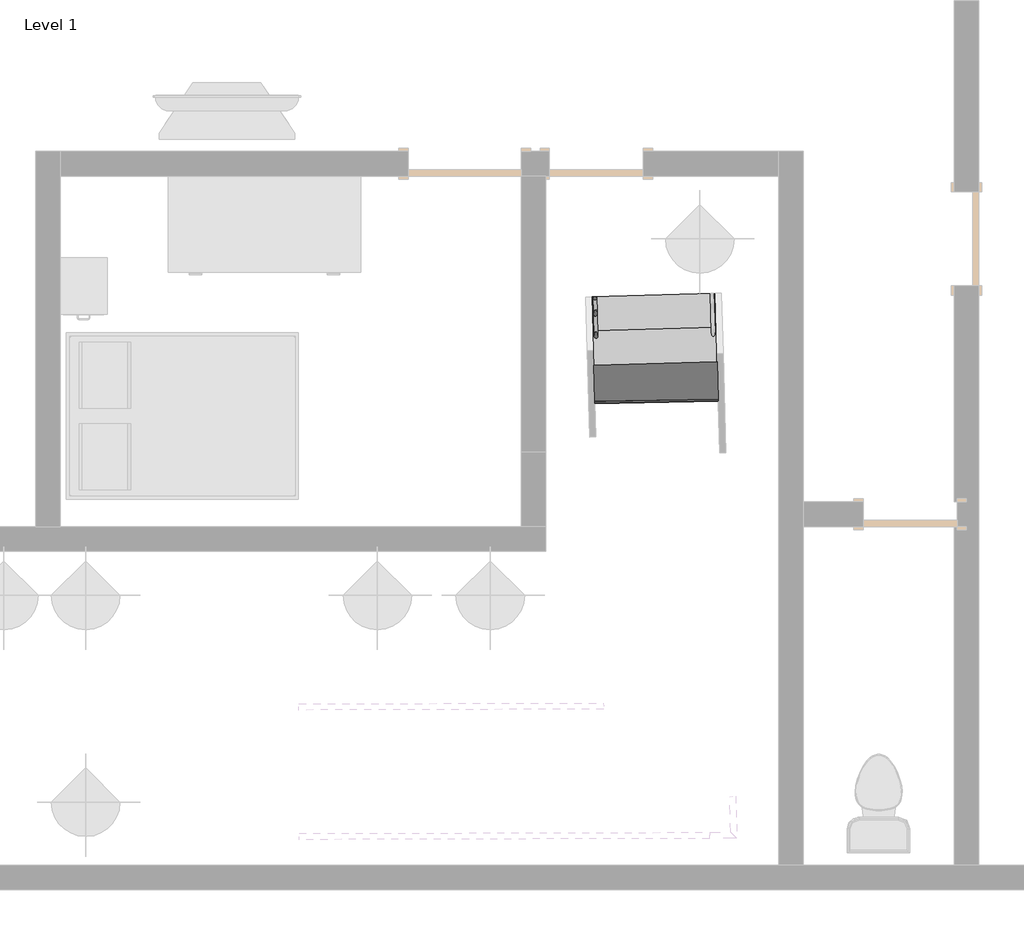
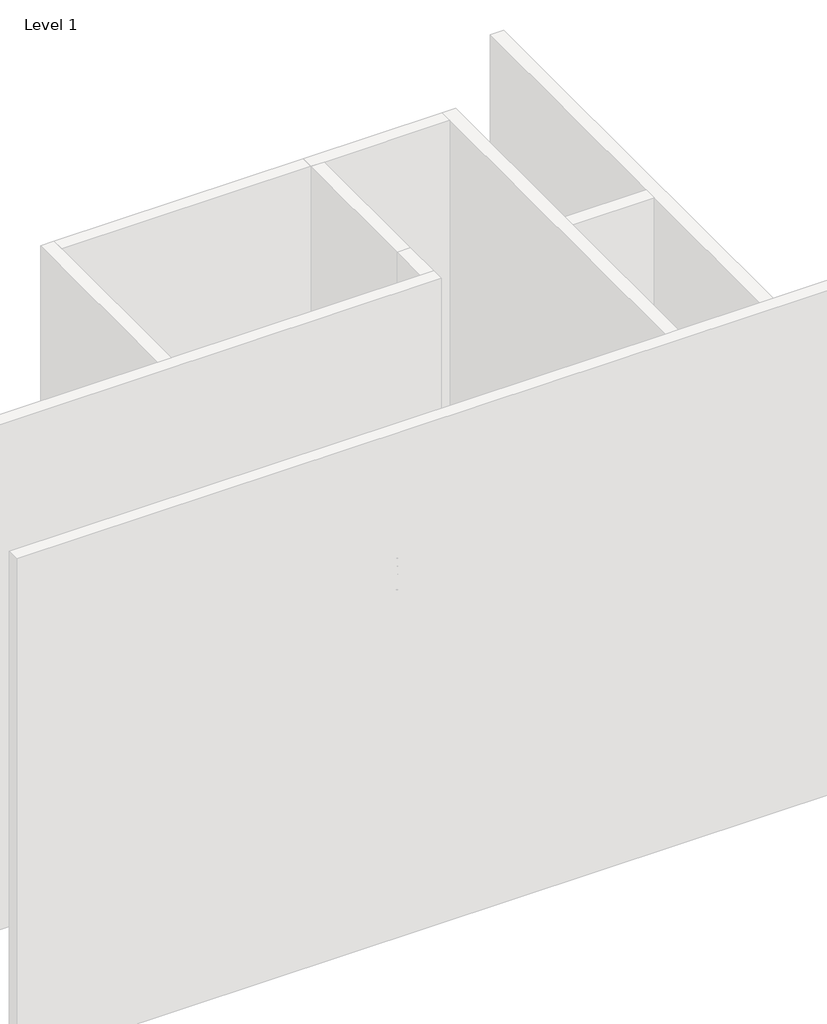
# One storey, part 3 of 4: 1 railing, 1 stair flight.
"""IFC4 building model written with IfcOpenShell, lengths in millimetres."""

from ifc_helpers import new_model, si_unit, point, frame, frame_2d, origin, place, context, project, spatial, circle_curve, ellipse_curve, trimmed, segment, composite_curve, outline, extrude, transform, mapped, element, save
from ifc_brep_helpers import plane_surface, cylinder_surface, advanced_brep
from components import stair_flight_50mm_tread_25mm_nosing_13mm_riser_f5a85d6c

model = new_model("IFC4")

# Units and contexts
model_context = context("Model", 3, world=origin())
ifc_project = project(units=[si_unit("LENGTHUNIT", "METRE", prefix="MILLI")], contexts=[model_context])

# Site, building, storey
site = spatial("IfcSite", under=ifc_project)
building = spatial("IfcBuilding", under=site)
storey = spatial("IfcBuildingStorey", under=building, Name="Level 1", Elevation=0.0)

# Railing
placement = place(None, origin())
element("IfcRailing", 1, ObjectType="900mm Pipe", at=placement, inside=storey, context=model_context, shape_type="SolidModel", body=[
    advanced_brep(
    [(2318.5093829, 1967.3130446, 1728.2894205), (2358.4929319, 1968.4601289, 1728.2894205), (2415.1133853, -1399.9817421, 4066.0870016), (2455.0969344, -1398.8346579, 4066.0870016)],
    [
        (0, 1, ellipse_curve(frame((2338.5011574, 1967.8865867, 1728.2894205), z_axis=(-0.028677106690059493, 0.9995887272032868, 0.0), x_axis=(0.0, 0.0, -1.0)), 24.3442691, 20.0)),
        (1, 0, ellipse_curve(frame((2338.5011574, 1967.8865867, 1728.2894205), z_axis=(-0.028677106690059493, 0.9995887272032868, 0.0), x_axis=(0.0, 0.0, -1.0)), 24.3442691, 20.0)),
        (2, 3, ellipse_curve(frame((2435.1051599, -1399.4082, 4066.0870016), z_axis=(0.013294885679998605, -0.46341557392153737, 0.8860413375580894), x_axis=(-0.025409101968956467, 0.885676932859188, 0.463606242557488)), 22.5723103, 20.0)),
        (3, 2, ellipse_curve(frame((2435.1051599, -1399.4082, 4066.0870016), z_axis=(0.013294885679998605, -0.46341557392153737, 0.8860413375580894), x_axis=(-0.025409101968956467, 0.885676932859188, 0.463606242557488)), 22.5723103, 20.0)),
        (0, 2),
        (3, 1),
    ],
    [
        plane_surface(frame((2338.5011574, 1967.8865867, 1752.6336896), z_axis=(-0.028677106690059493, 0.9995887272032868, 0.0), x_axis=(0.9995887272032868, 0.028677106690059493, 0.0))),
        plane_surface(frame((2434.5316177, -1379.4164255, 4076.5516656), z_axis=(0.013294885679998605, -0.46341557392153737, 0.8860413375580894), x_axis=(0.9999116191017864, 0.006161601645505646, -0.01178085949353162))),
        cylinder_surface(frame((2338.8281559, 1956.4885063, 1736.2027178), z_axis=(-0.023559636581175762, 0.8212107099253749, -0.5701385037234595), x_axis=(0.999588727203287, 0.028677106690059496, 0.0)), 20.0),
    ],
    [
        (0, [[1, 2]]),
        (1, [[3, 4]]),
        (2, [[-1, 5, -4, 6]]),
        (2, [[-2, -6, -3, -5]]),
    ],
),
    advanced_brep(
    [(2415.2157347, -1403.5493025, 4064.2195676), (2455.1992838, -1402.4022182, 4064.2195676), (2415.2157347, -1403.5493025, 4120.8684951), (2455.1992838, -1402.4022182, 4141.2378675)],
    [
        (0, 1, ellipse_curve(frame((2435.2075093, -1402.9757604, 4064.2195676), z_axis=(-0.013294885679998605, 0.46341557392153737, -0.8860413375580894), x_axis=(0.02540910196895648, -0.8856769328591886, -0.46360624255748706)), 22.5723103, 20.0)),
        (1, 0, ellipse_curve(frame((2435.2075093, -1402.9757604, 4064.2195676), z_axis=(-0.013294885679998605, 0.46341557392153737, -0.8860413375580894), x_axis=(0.02540910196895648, -0.8856769328591886, -0.46360624255748706)), 22.5723103, 20.0)),
        (2, 3, ellipse_curve(frame((2435.2075093, -1402.9757604, 4131.0531813), z_axis=(-0.4539050357854136, -0.0012028713064138657, 0.8910492531781073), x_axis=(-0.8910461243784461, -0.002361317304725111, -0.4539066296175206)), 22.4454484, 20.0)),
        (3, 2, ellipse_curve(frame((2435.2075093, -1402.9757604, 4131.0531813), z_axis=(-0.4539050357854136, -0.0012028713064138657, 0.8910492531781073), x_axis=(-0.8910461243784461, -0.002361317304725111, -0.4539066296175206)), 22.4454484, 20.0)),
        (0, 2),
        (3, 1),
    ],
    [
        plane_surface(frame((2435.1051599, -1399.4082, 4066.0870016), z_axis=(-0.013294885679998605, 0.46341557392153737, -0.8860413375580894), x_axis=(0.9999116191017864, 0.006161601645505646, -0.01178085949353162))),
        plane_surface(frame((2435.1051599, -1399.4082, 4131.00586), z_axis=(-0.4539050357854136, -0.0012028713064138657, 0.8910492531781073), x_axis=(0.8910500650853702, -0.000612748222324323, 0.45390462219608824))),
        cylinder_surface(frame((2435.2075093, -1402.9757604, 4066.0870016), z_axis=(0.0, 0.0, -1.0), x_axis=(0.9995887272032868, 0.028677106690059573, 0.0)), 20.0),
    ],
    [
        (0, [[1, 2]]),
        (1, [[3, 4]]),
        (2, [[-1, 5, -4, 6]]),
        (2, [[-2, -6, -3, -5]]),
    ],
),
    advanced_brep(
    [(2435.052159, -1379.4082702, 4131.00586), (2435.1581607, -1419.4081298, 4131.00586), (-60.3127324, -1386.0211134, 5944.7187793), (-60.2067307, -1426.020973, 5944.7187793)],
    [
        (0, 1, ellipse_curve(frame((2435.1051599, -1399.4082, 4131.00586), z_axis=(0.4539050357854136, 0.0012028713064138657, -0.8910492531781073), x_axis=(0.8910461243784458, 0.002361317304725109, 0.4539066296175212)), 22.4454484, 20.0)),
        (1, 0, ellipse_curve(frame((2435.1051599, -1399.4082, 4131.00586), z_axis=(0.4539050357854136, 0.0012028713064138657, -0.8910492531781073), x_axis=(0.8910461243784458, 0.002361317304725109, 0.4539066296175212)), 22.4454484, 20.0)),
        (2, 3, ellipse_curve(frame((-60.2597316, -1406.0210432, 5944.7187793), z_axis=(-0.9999964886344385, -0.0026500412814528056, 0.0), x_axis=(0.0, 0.0, -1.0)), 24.7247417, 20.0)),
        (3, 2, ellipse_curve(frame((-60.2597316, -1406.0210432, 5944.7187793), z_axis=(-0.9999964886344385, -0.0026500412814528056, 0.0), x_axis=(0.0, 0.0, -1.0)), 24.7247417, 20.0)),
        (0, 2),
        (3, 1),
    ],
    [
        plane_surface(frame((2455.1050896, -1399.3551992, 4141.1939978), z_axis=(0.4539050357854136, 0.0012028713064138657, -0.8910492531781073), x_axis=(0.8910500650853702, -0.000612748222324323, 0.45390462219608824))),
        plane_surface(frame((-60.2597316, -1406.0210432, 5969.443521), z_axis=(-0.9999964886344385, -0.0026500412814528056, 0.0), x_axis=(0.0026500412814528056, -0.9999964886344385, 0.0))),
        cylinder_surface(frame((2443.3463801, -1399.3863604, 4125.0158713), z_axis=(0.8089034863007496, 0.0021436351584947526, -0.5879375431785253), x_axis=(0.0026500412814528056, -0.9999964886344385, 0.0)), 20.0),
    ],
    [
        (0, [[1, 2]]),
        (1, [[3, 4]]),
        (2, [[-1, 5, -4, 6]]),
        (2, [[-2, -6, -3, -5]]),
    ],
),
    advanced_brep(
    [(2353.4949883, 1968.3167433, 1609.3754878), (2323.5073265, 1967.4564301, 1609.3754878), (2449.6798883, -1384.3695236, 3937.0308733), (2419.6698266, -1384.4490517, 3936.488801)],
    [
        (0, 1, ellipse_curve(frame((2338.5011574, 1967.8865867, 1609.3754878), z_axis=(-0.028677106690059493, 0.9995887272032868, 0.0), x_axis=(0.0, 0.0, -1.0)), 18.2582019, 15.0)),
        (1, 0, ellipse_curve(frame((2338.5011574, 1967.8865867, 1609.3754878), z_axis=(-0.028677106690059493, 0.9995887272032868, 0.0), x_axis=(0.0, 0.0, -1.0)), 18.2582019, 15.0)),
        (2, 3, ellipse_curve(frame((2434.6748575, -1384.4092877, 3936.7598372), z_axis=(0.0026500412814528056, -0.9999964886344385, 0.0), x_axis=(-0.037478985760625305, -9.93212082056486e-05, -0.9992974110652206)), 18.2643896, 15.0)),
        (3, 2, ellipse_curve(frame((2434.6748575, -1384.4092877, 3936.7598372), z_axis=(0.0026500412814528056, -0.9999964886344385, 0.0), x_axis=(-0.037478985760625305, -9.93212082056486e-05, -0.9992974110652206)), 18.2643896, 15.0)),
        (0, 2),
        (3, 1),
    ],
    [
        plane_surface(frame((2338.5011574, 1967.8865867, 1627.6336896), z_axis=(-0.028677106690059493, 0.9995887272032868, 0.0), x_axis=(0.9995887272032868, 0.028677106690059493, 0.0))),
        plane_surface(frame((2434.6748575, -1384.4092877, 3955.018039), z_axis=(0.0026500412814528056, -0.9999964886344385, 0.0), x_axis=(0.9999964886344385, 0.0026500412814528056, 0.0))),
        cylinder_surface(frame((2338.7464062, 1959.3380264, 1615.3104608), z_axis=(-0.023559636581175762, 0.8212107099253748, -0.5701385037234593), x_axis=(-0.9995887272032868, -0.028677106690059496, 0.0)), 15.0),
    ],
    [
        (0, [[1, 2]]),
        (1, [[3, 4]]),
        (2, [[-1, 5, -4, 6]]),
        (2, [[-2, -6, -3, -5]]),
    ],
),
    advanced_brep(
    [(2450.5404931, -1414.3673483, 4000.9970318), (2449.6798883, -1384.3695236, 4001.5647634), (-60.219981, -1421.0209905, 5825.8999647), (-60.2994822, -1391.0210959, 5825.8999647)],
    [
        (0, 1, ellipse_curve(frame((2450.1101907, -1399.3684359, 4001.2808976), z_axis=(0.9995887272032868, 0.028677106690059493, 0.0), x_axis=(0.0010262798280310235, -0.03577270741234457, -0.9993594249088289)), 18.5498407, 15.0)),
        (1, 0, ellipse_curve(frame((2450.1101907, -1399.3684359, 4001.2808976), z_axis=(0.9995887272032868, 0.028677106690059493, 0.0), x_axis=(0.0010262798280310235, -0.03577270741234457, -0.9993594249088289)), 18.5498407, 15.0)),
        (2, 3, ellipse_curve(frame((-60.2597316, -1406.0210432, 5825.8999647), z_axis=(-0.9999964886344385, -0.0026500412814528056, 0.0), x_axis=(0.0, 0.0, -1.0)), 18.5435563, 15.0)),
        (3, 2, ellipse_curve(frame((-60.2597316, -1406.0210432, 5825.8999647), z_axis=(-0.9999964886344385, -0.0026500412814528056, 0.0), x_axis=(0.0, 0.0, -1.0)), 18.5435563, 15.0)),
        (0, 2),
        (3, 1),
    ],
    [
        plane_surface(frame((2450.1101907, -1399.3684359, 4019.8244539), z_axis=(0.9995887272032868, 0.028677106690059493, 0.0), x_axis=(0.028677106690059493, -0.9995887272032868, 0.0))),
        plane_surface(frame((-60.2597316, -1406.0210432, 5844.443521), z_axis=(-0.9999964886344385, -0.0026500412814528056, 0.0), x_axis=(0.0026500412814528056, -0.9999964886344385, 0.0))),
        cylinder_surface(frame((2441.2911585, -1399.3918068, 4007.690859), z_axis=(0.8089034863007496, 0.0021436351584947526, -0.5879375431785254), x_axis=(-0.0026500412814528056, 0.9999964886344385, 0.0)), 15.0),
    ],
    [
        (0, [[1, 2]]),
        (1, [[3, 4]]),
        (2, [[-1, 5, -4, 6]]),
        (2, [[-2, -6, -3, -5]]),
    ],
),
    advanced_brep(
    [(2353.4949883, 1968.3167433, 1484.3754878), (2323.5073265, 1967.4564301, 1484.3754878), (2449.6798883, -1384.3695236, 3812.0308733), (2419.6698266, -1384.4490517, 3811.488801)],
    [
        (0, 1, ellipse_curve(frame((2338.5011574, 1967.8865867, 1484.3754878), z_axis=(-0.028677106690059493, 0.9995887272032868, 0.0), x_axis=(0.0, 0.0, -1.0)), 18.2582019, 15.0)),
        (1, 0, ellipse_curve(frame((2338.5011574, 1967.8865867, 1484.3754878), z_axis=(-0.028677106690059493, 0.9995887272032868, 0.0), x_axis=(0.0, 0.0, -1.0)), 18.2582019, 15.0)),
        (2, 3, ellipse_curve(frame((2434.6748575, -1384.4092877, 3811.7598372), z_axis=(0.0026500412814528056, -0.9999964886344385, 0.0), x_axis=(-0.037478985760625305, -9.93212082056486e-05, -0.9992974110652206)), 18.2643896, 15.0)),
        (3, 2, ellipse_curve(frame((2434.6748575, -1384.4092877, 3811.7598372), z_axis=(0.0026500412814528056, -0.9999964886344385, 0.0), x_axis=(-0.037478985760625305, -9.93212082056486e-05, -0.9992974110652206)), 18.2643896, 15.0)),
        (0, 2),
        (3, 1),
    ],
    [
        plane_surface(frame((2338.5011574, 1967.8865867, 1502.6336896), z_axis=(-0.028677106690059493, 0.9995887272032868, 0.0), x_axis=(0.9995887272032868, 0.028677106690059493, 0.0))),
        plane_surface(frame((2434.6748575, -1384.4092877, 3830.018039), z_axis=(0.0026500412814528056, -0.9999964886344385, 0.0), x_axis=(0.9999964886344385, 0.0026500412814528056, 0.0))),
        cylinder_surface(frame((2338.7464062, 1959.3380264, 1490.3104608), z_axis=(-0.023559636581175762, 0.8212107099253748, -0.5701385037234593), x_axis=(-0.9995887272032868, -0.028677106690059496, 0.0)), 15.0),
    ],
    [
        (0, [[1, 2]]),
        (1, [[3, 4]]),
        (2, [[-1, 5, -4, 6]]),
        (2, [[-2, -6, -3, -5]]),
    ],
),
    advanced_brep(
    [(2450.5404931, -1414.3673483, 3875.9970318), (2449.6798883, -1384.3695236, 3876.5647634), (-60.219981, -1421.0209905, 5700.8999647), (-60.2994822, -1391.0210959, 5700.8999647)],
    [
        (0, 1, ellipse_curve(frame((2450.1101907, -1399.3684359, 3876.2808976), z_axis=(0.9995887272032868, 0.028677106690059493, 0.0), x_axis=(0.001026279828031024, -0.03577270741234459, -0.9993594249088289)), 18.5498407, 15.0)),
        (1, 0, ellipse_curve(frame((2450.1101907, -1399.3684359, 3876.2808976), z_axis=(0.9995887272032868, 0.028677106690059493, 0.0), x_axis=(0.001026279828031024, -0.03577270741234459, -0.9993594249088289)), 18.5498407, 15.0)),
        (2, 3, ellipse_curve(frame((-60.2597316, -1406.0210432, 5700.8999647), z_axis=(-0.9999964886344385, -0.0026500412814528056, 0.0), x_axis=(0.0, 0.0, -0.9999999999999999)), 18.5435563, 15.0)),
        (3, 2, ellipse_curve(frame((-60.2597316, -1406.0210432, 5700.8999647), z_axis=(-0.9999964886344385, -0.0026500412814528056, 0.0), x_axis=(0.0, 0.0, -0.9999999999999999)), 18.5435563, 15.0)),
        (0, 2),
        (3, 1),
    ],
    [
        plane_surface(frame((2450.1101907, -1399.3684359, 3894.8244539), z_axis=(0.9995887272032868, 0.028677106690059493, 0.0), x_axis=(0.028677106690059493, -0.9995887272032868, 0.0))),
        plane_surface(frame((-60.2597316, -1406.0210432, 5719.443521), z_axis=(-0.9999964886344385, -0.0026500412814528056, 0.0), x_axis=(0.0026500412814528056, -0.9999964886344385, 0.0))),
        cylinder_surface(frame((2441.2911585, -1399.3918068, 3882.690859), z_axis=(0.8089034863007497, 0.0021436351584947534, -0.5879375431785252), x_axis=(-0.002650041281452806, 0.9999964886344385, 0.0)), 15.0),
    ],
    [
        (0, [[1, 2]]),
        (1, [[3, 4]]),
        (2, [[-1, 5, -4, 6]]),
        (2, [[-2, -6, -3, -5]]),
    ],
),
    advanced_brep(
    [(2353.4949883, 1968.3167433, 1359.3754878), (2323.5073265, 1967.4564301, 1359.3754878), (2449.6798883, -1384.3695236, 3687.0308733), (2419.6698266, -1384.4490517, 3686.488801)],
    [
        (0, 1, ellipse_curve(frame((2338.5011574, 1967.8865867, 1359.3754878), z_axis=(-0.028677106690059493, 0.9995887272032868, 0.0), x_axis=(0.0, 0.0, -1.0)), 18.2582019, 15.0)),
        (1, 0, ellipse_curve(frame((2338.5011574, 1967.8865867, 1359.3754878), z_axis=(-0.028677106690059493, 0.9995887272032868, 0.0), x_axis=(0.0, 0.0, -1.0)), 18.2582019, 15.0)),
        (2, 3, ellipse_curve(frame((2434.6748575, -1384.4092877, 3686.7598372), z_axis=(0.0026500412814528056, -0.9999964886344385, 0.0), x_axis=(-0.03747898576062528, -9.932120820564857e-05, -0.9992974110652205)), 18.2643896, 15.0)),
        (3, 2, ellipse_curve(frame((2434.6748575, -1384.4092877, 3686.7598372), z_axis=(0.0026500412814528056, -0.9999964886344385, 0.0), x_axis=(-0.03747898576062528, -9.932120820564857e-05, -0.9992974110652205)), 18.2643896, 15.0)),
        (0, 2),
        (3, 1),
    ],
    [
        plane_surface(frame((2338.5011574, 1967.8865867, 1377.6336896), z_axis=(-0.028677106690059493, 0.9995887272032868, 0.0), x_axis=(0.9995887272032868, 0.028677106690059493, 0.0))),
        plane_surface(frame((2434.6748575, -1384.4092877, 3705.018039), z_axis=(0.0026500412814528056, -0.9999964886344385, 0.0), x_axis=(0.9999964886344385, 0.0026500412814528056, 0.0))),
        cylinder_surface(frame((2338.7464062, 1959.3380264, 1365.3104608), z_axis=(-0.023559636581175762, 0.8212107099253749, -0.5701385037234595), x_axis=(-0.999588727203287, -0.028677106690059496, 0.0)), 15.0),
    ],
    [
        (0, [[1, 2]]),
        (1, [[3, 4]]),
        (2, [[-1, 5, -4, 6]]),
        (2, [[-2, -6, -3, -5]]),
    ],
),
    advanced_brep(
    [(2450.5404931, -1414.3673483, 3750.9970318), (2449.6798883, -1384.3695236, 3751.5647634), (-60.219981, -1421.0209905, 5575.8999647), (-60.2994822, -1391.0210959, 5575.8999647)],
    [
        (0, 1, ellipse_curve(frame((2450.1101907, -1399.3684359, 3751.2808976), z_axis=(0.9995887272032868, 0.028677106690059493, 0.0), x_axis=(0.001026279828031024, -0.03577270741234459, -0.9993594249088289)), 18.5498407, 15.0)),
        (1, 0, ellipse_curve(frame((2450.1101907, -1399.3684359, 3751.2808976), z_axis=(0.9995887272032868, 0.028677106690059493, 0.0), x_axis=(0.001026279828031024, -0.03577270741234459, -0.9993594249088289)), 18.5498407, 15.0)),
        (2, 3, ellipse_curve(frame((-60.2597316, -1406.0210432, 5575.8999647), z_axis=(-0.9999964886344385, -0.0026500412814528056, 0.0), x_axis=(0.0, 0.0, -0.9999999999999999)), 18.5435563, 15.0)),
        (3, 2, ellipse_curve(frame((-60.2597316, -1406.0210432, 5575.8999647), z_axis=(-0.9999964886344385, -0.0026500412814528056, 0.0), x_axis=(0.0, 0.0, -0.9999999999999999)), 18.5435563, 15.0)),
        (0, 2),
        (3, 1),
    ],
    [
        plane_surface(frame((2450.1101907, -1399.3684359, 3769.8244539), z_axis=(0.9995887272032868, 0.028677106690059493, 0.0), x_axis=(0.028677106690059493, -0.9995887272032868, 0.0))),
        plane_surface(frame((-60.2597316, -1406.0210432, 5594.443521), z_axis=(-0.9999964886344385, -0.0026500412814528056, 0.0), x_axis=(0.0026500412814528056, -0.9999964886344385, 0.0))),
        cylinder_surface(frame((2441.2911585, -1399.3918068, 3757.690859), z_axis=(0.8089034863007497, 0.0021436351584947534, -0.5879375431785252), x_axis=(-0.002650041281452806, 0.9999964886344385, 0.0)), 15.0),
    ],
    [
        (0, [[1, 2]]),
        (1, [[3, 4]]),
        (2, [[-1, 5, -4, 6]]),
        (2, [[-2, -6, -3, -5]]),
    ],
),
    advanced_brep(
    [(2353.4949883, 1968.3167433, 1234.3754878), (2323.5073265, 1967.4564301, 1234.3754878), (2449.6798883, -1384.3695236, 3562.0308733), (2419.6698266, -1384.4490517, 3561.488801)],
    [
        (0, 1, ellipse_curve(frame((2338.5011574, 1967.8865867, 1234.3754878), z_axis=(-0.028677106690059493, 0.9995887272032868, 0.0), x_axis=(0.0, 0.0, -1.0)), 18.2582019, 15.0)),
        (1, 0, ellipse_curve(frame((2338.5011574, 1967.8865867, 1234.3754878), z_axis=(-0.028677106690059493, 0.9995887272032868, 0.0), x_axis=(0.0, 0.0, -1.0)), 18.2582019, 15.0)),
        (2, 3, ellipse_curve(frame((2434.6748575, -1384.4092877, 3561.7598372), z_axis=(0.0026500412814528056, -0.9999964886344385, 0.0), x_axis=(-0.037478985760625305, -9.93212082056486e-05, -0.9992974110652206)), 18.2643896, 15.0)),
        (3, 2, ellipse_curve(frame((2434.6748575, -1384.4092877, 3561.7598372), z_axis=(0.0026500412814528056, -0.9999964886344385, 0.0), x_axis=(-0.037478985760625305, -9.93212082056486e-05, -0.9992974110652206)), 18.2643896, 15.0)),
        (0, 2),
        (3, 1),
    ],
    [
        plane_surface(frame((2338.5011574, 1967.8865867, 1252.6336896), z_axis=(-0.028677106690059493, 0.9995887272032868, 0.0), x_axis=(0.9995887272032868, 0.028677106690059493, 0.0))),
        plane_surface(frame((2434.6748575, -1384.4092877, 3580.018039), z_axis=(0.0026500412814528056, -0.9999964886344385, 0.0), x_axis=(0.9999964886344385, 0.0026500412814528056, 0.0))),
        cylinder_surface(frame((2338.7464062, 1959.3380264, 1240.3104608), z_axis=(-0.023559636581175762, 0.8212107099253748, -0.5701385037234593), x_axis=(-0.9995887272032868, -0.028677106690059496, 0.0)), 15.0),
    ],
    [
        (0, [[1, 2]]),
        (1, [[3, 4]]),
        (2, [[-1, 5, -4, 6]]),
        (2, [[-2, -6, -3, -5]]),
    ],
),
    advanced_brep(
    [(2450.5404931, -1414.3673483, 3625.9970318), (2449.6798883, -1384.3695236, 3626.5647634), (-60.219981, -1421.0209905, 5450.8999647), (-60.2994822, -1391.0210959, 5450.8999647)],
    [
        (0, 1, ellipse_curve(frame((2450.1101907, -1399.3684359, 3626.2808976), z_axis=(0.9995887272032868, 0.028677106690059493, 0.0), x_axis=(0.0010262798280310237, -0.03577270741234458, -0.999359424908829)), 18.5498407, 15.0)),
        (1, 0, ellipse_curve(frame((2450.1101907, -1399.3684359, 3626.2808976), z_axis=(0.9995887272032868, 0.028677106690059493, 0.0), x_axis=(0.0010262798280310237, -0.03577270741234458, -0.999359424908829)), 18.5498407, 15.0)),
        (2, 3, ellipse_curve(frame((-60.2597316, -1406.0210432, 5450.8999647), z_axis=(-0.9999964886344385, -0.0026500412814528056, 0.0), x_axis=(0.0, 0.0, -1.0)), 18.5435563, 15.0)),
        (3, 2, ellipse_curve(frame((-60.2597316, -1406.0210432, 5450.8999647), z_axis=(-0.9999964886344385, -0.0026500412814528056, 0.0), x_axis=(0.0, 0.0, -1.0)), 18.5435563, 15.0)),
        (0, 2),
        (3, 1),
    ],
    [
        plane_surface(frame((2450.1101907, -1399.3684359, 3644.8244539), z_axis=(0.9995887272032868, 0.028677106690059493, 0.0), x_axis=(0.028677106690059493, -0.9995887272032868, 0.0))),
        plane_surface(frame((-60.2597316, -1406.0210432, 5469.443521), z_axis=(-0.9999964886344385, -0.0026500412814528056, 0.0), x_axis=(0.0026500412814528056, -0.9999964886344385, 0.0))),
        cylinder_surface(frame((2441.2911585, -1399.3918068, 3632.690859), z_axis=(0.8089034863007496, 0.0021436351584947526, -0.5879375431785253), x_axis=(-0.0026500412814528056, 0.9999964886344385, 0.0)), 15.0),
    ],
    [
        (0, [[1, 2]]),
        (1, [[3, 4]]),
        (2, [[-1, 5, -4, 6]]),
        (2, [[-2, -6, -3, -5]]),
    ],
),
    advanced_brep(
    [(2353.4949883, 1968.3167433, 1109.3754878), (2323.5073265, 1967.4564301, 1109.3754878), (2449.6798883, -1384.3695236, 3437.0308733), (2419.6698266, -1384.4490517, 3436.488801)],
    [
        (0, 1, ellipse_curve(frame((2338.5011574, 1967.8865867, 1109.3754878), z_axis=(-0.028677106690059493, 0.9995887272032868, 0.0), x_axis=(0.0, 0.0, -1.0)), 18.2582019, 15.0)),
        (1, 0, ellipse_curve(frame((2338.5011574, 1967.8865867, 1109.3754878), z_axis=(-0.028677106690059493, 0.9995887272032868, 0.0), x_axis=(0.0, 0.0, -1.0)), 18.2582019, 15.0)),
        (2, 3, ellipse_curve(frame((2434.6748575, -1384.4092877, 3436.7598372), z_axis=(0.0026500412814528056, -0.9999964886344385, 0.0), x_axis=(-0.037478985760625305, -9.93212082056486e-05, -0.9992974110652206)), 18.2643896, 15.0)),
        (3, 2, ellipse_curve(frame((2434.6748575, -1384.4092877, 3436.7598372), z_axis=(0.0026500412814528056, -0.9999964886344385, 0.0), x_axis=(-0.037478985760625305, -9.93212082056486e-05, -0.9992974110652206)), 18.2643896, 15.0)),
        (0, 2),
        (3, 1),
    ],
    [
        plane_surface(frame((2338.5011574, 1967.8865867, 1127.6336896), z_axis=(-0.028677106690059493, 0.9995887272032868, 0.0), x_axis=(0.9995887272032868, 0.028677106690059493, 0.0))),
        plane_surface(frame((2434.6748575, -1384.4092877, 3455.018039), z_axis=(0.0026500412814528056, -0.9999964886344385, 0.0), x_axis=(0.9999964886344385, 0.0026500412814528056, 0.0))),
        cylinder_surface(frame((2338.7464062, 1959.3380264, 1115.3104608), z_axis=(-0.023559636581175762, 0.8212107099253748, -0.5701385037234593), x_axis=(-0.9995887272032868, -0.028677106690059496, 0.0)), 15.0),
    ],
    [
        (0, [[1, 2]]),
        (1, [[3, 4]]),
        (2, [[-1, 5, -4, 6]]),
        (2, [[-2, -6, -3, -5]]),
    ],
),
    advanced_brep(
    [(2450.5404931, -1414.3673483, 3500.9970318), (2449.6798883, -1384.3695236, 3501.5647634), (-60.219981, -1421.0209905, 5325.8999647), (-60.2994822, -1391.0210959, 5325.8999647)],
    [
        (0, 1, ellipse_curve(frame((2450.1101907, -1399.3684359, 3501.2808976), z_axis=(0.9995887272032868, 0.028677106690059493, 0.0), x_axis=(0.0010262798280310235, -0.03577270741234457, -0.9993594249088289)), 18.5498407, 15.0)),
        (1, 0, ellipse_curve(frame((2450.1101907, -1399.3684359, 3501.2808976), z_axis=(0.9995887272032868, 0.028677106690059493, 0.0), x_axis=(0.0010262798280310235, -0.03577270741234457, -0.9993594249088289)), 18.5498407, 15.0)),
        (2, 3, ellipse_curve(frame((-60.2597316, -1406.0210432, 5325.8999647), z_axis=(-0.9999964886344385, -0.0026500412814528056, 0.0), x_axis=(0.0, 0.0, -1.0)), 18.5435563, 15.0)),
        (3, 2, ellipse_curve(frame((-60.2597316, -1406.0210432, 5325.8999647), z_axis=(-0.9999964886344385, -0.0026500412814528056, 0.0), x_axis=(0.0, 0.0, -1.0)), 18.5435563, 15.0)),
        (0, 2),
        (3, 1),
    ],
    [
        plane_surface(frame((2450.1101907, -1399.3684359, 3519.8244539), z_axis=(0.9995887272032868, 0.028677106690059493, 0.0), x_axis=(0.028677106690059493, -0.9995887272032868, 0.0))),
        plane_surface(frame((-60.2597316, -1406.0210432, 5344.443521), z_axis=(-0.9999964886344385, -0.0026500412814528056, 0.0), x_axis=(0.0026500412814528056, -0.9999964886344385, 0.0))),
        cylinder_surface(frame((2441.2911585, -1399.3918068, 3507.690859), z_axis=(0.8089034863007496, 0.0021436351584947526, -0.5879375431785254), x_axis=(-0.0026500412814528056, 0.9999964886344385, 0.0)), 15.0),
    ],
    [
        (0, [[1, 2]]),
        (1, [[3, 4]]),
        (2, [[-1, 5, -4, 6]]),
        (2, [[-2, -6, -3, -5]]),
    ],
),
    advanced_brep(
    [(2353.4949883, 1968.3167433, 984.3754878), (2323.5073265, 1967.4564301, 984.3754878), (2449.6798883, -1384.3695236, 3312.0308733), (2419.6698266, -1384.4490517, 3311.488801)],
    [
        (0, 1, ellipse_curve(frame((2338.5011574, 1967.8865867, 984.3754878), z_axis=(-0.028677106690059493, 0.9995887272032868, 0.0), x_axis=(0.0, 0.0, -1.0)), 18.2582019, 15.0)),
        (1, 0, ellipse_curve(frame((2338.5011574, 1967.8865867, 984.3754878), z_axis=(-0.028677106690059493, 0.9995887272032868, 0.0), x_axis=(0.0, 0.0, -1.0)), 18.2582019, 15.0)),
        (2, 3, ellipse_curve(frame((2434.6748575, -1384.4092877, 3311.7598372), z_axis=(0.0026500412814528056, -0.9999964886344385, 0.0), x_axis=(-0.037478985760625305, -9.93212082056486e-05, -0.9992974110652206)), 18.2643896, 15.0)),
        (3, 2, ellipse_curve(frame((2434.6748575, -1384.4092877, 3311.7598372), z_axis=(0.0026500412814528056, -0.9999964886344385, 0.0), x_axis=(-0.037478985760625305, -9.93212082056486e-05, -0.9992974110652206)), 18.2643896, 15.0)),
        (0, 2),
        (3, 1),
    ],
    [
        plane_surface(frame((2338.5011574, 1967.8865867, 1002.6336896), z_axis=(-0.028677106690059493, 0.9995887272032868, 0.0), x_axis=(0.9995887272032868, 0.028677106690059493, 0.0))),
        plane_surface(frame((2434.6748575, -1384.4092877, 3330.018039), z_axis=(0.0026500412814528056, -0.9999964886344385, 0.0), x_axis=(0.9999964886344385, 0.0026500412814528056, 0.0))),
        cylinder_surface(frame((2338.7464062, 1959.3380264, 990.3104608), z_axis=(-0.023559636581175762, 0.8212107099253748, -0.5701385037234593), x_axis=(-0.9995887272032868, -0.028677106690059496, 0.0)), 15.0),
    ],
    [
        (0, [[1, 2]]),
        (1, [[3, 4]]),
        (2, [[-1, 5, -4, 6]]),
        (2, [[-2, -6, -3, -5]]),
    ],
),
    advanced_brep(
    [(2450.5404931, -1414.3673483, 3375.9970318), (2449.6798883, -1384.3695236, 3376.5647634), (-60.219981, -1421.0209905, 5200.8999647), (-60.2994822, -1391.0210959, 5200.8999647)],
    [
        (0, 1, ellipse_curve(frame((2450.1101907, -1399.3684359, 3376.2808976), z_axis=(0.9995887272032868, 0.028677106690059493, 0.0), x_axis=(0.0010262798280310235, -0.03577270741234457, -0.9993594249088289)), 18.5498407, 15.0)),
        (1, 0, ellipse_curve(frame((2450.1101907, -1399.3684359, 3376.2808976), z_axis=(0.9995887272032868, 0.028677106690059493, 0.0), x_axis=(0.0010262798280310235, -0.03577270741234457, -0.9993594249088289)), 18.5498407, 15.0)),
        (2, 3, ellipse_curve(frame((-60.2597316, -1406.0210432, 5200.8999647), z_axis=(-0.9999964886344385, -0.0026500412814528056, 0.0), x_axis=(0.0, 0.0, -1.0)), 18.5435563, 15.0)),
        (3, 2, ellipse_curve(frame((-60.2597316, -1406.0210432, 5200.8999647), z_axis=(-0.9999964886344385, -0.0026500412814528056, 0.0), x_axis=(0.0, 0.0, -1.0)), 18.5435563, 15.0)),
        (0, 2),
        (3, 1),
    ],
    [
        plane_surface(frame((2450.1101907, -1399.3684359, 3394.8244539), z_axis=(0.9995887272032868, 0.028677106690059493, 0.0), x_axis=(0.028677106690059493, -0.9995887272032868, 0.0))),
        plane_surface(frame((-60.2597316, -1406.0210432, 5219.443521), z_axis=(-0.9999964886344385, -0.0026500412814528056, 0.0), x_axis=(0.0026500412814528056, -0.9999964886344385, 0.0))),
        cylinder_surface(frame((2441.2911585, -1399.3918068, 3382.690859), z_axis=(0.8089034863007496, 0.0021436351584947526, -0.5879375431785254), x_axis=(-0.0026500412814528056, 0.9999964886344385, 0.0)), 15.0),
    ],
    [
        (0, [[1, 2]]),
        (1, [[3, 4]]),
        (2, [[-1, 5, -4, 6]]),
        (2, [[-2, -6, -3, -5]]),
    ],
),
    advanced_brep(
    [(435.0790571, -1392.2083265, 5559.9415083), (435.0790571, -1392.2083265, 4695.6521739), (435.1453081, -1417.2082387, 4695.6521739), (435.1453081, -1417.2082387, 5559.9415083)],
    [
        (0, 1),
        (1, 2, circle_curve(frame((435.1121826, -1404.7082826, 4695.6521739), z_axis=(0.0, 0.0, 1.0), x_axis=(0.002650041281452805, -0.9999964886344386, 0.0)), 12.5)),
        (2, 3),
        (3, 0, ellipse_curve(frame((435.1121826, -1404.7082826, 5559.9415083), z_axis=(-0.5879354787148848, -0.0015580587603390356, -0.808906326666567), x_axis=(-0.8089034863007493, -0.0021436351584947512, 0.587937543178526)), 15.4529636, 12.5)),
        (0, 3, ellipse_curve(frame((435.1121826, -1404.7082826, 5559.9415083), z_axis=(-0.5879354787148848, -0.0015580587603390356, -0.808906326666567), x_axis=(-0.8089034863007493, -0.0021436351584947512, 0.587937543178526)), 15.4529636, 12.5)),
        (2, 1, circle_curve(frame((435.1121826, -1404.7082826, 4695.6521739), z_axis=(0.0, 0.0, 1.0), x_axis=(0.002650041281452805, -0.9999964886344386, 0.0)), 12.5)),
    ],
    [
        cylinder_surface(frame((435.1121826, -1404.7082826, 4595.6521739), z_axis=(0.0, 0.0, 1.0), x_axis=(0.002650041281452805, -0.9999964886344386, 0.0)), 12.5),
        plane_surface(frame((410.1785214, -1429.7744458, 5578.1122632), z_axis=(0.5879354787148848, 0.0015580587603390356, 0.808906326666567), x_axis=(-0.002650041281452805, 0.9999964886344386, 0.0))),
        plane_surface(frame((460.1783458, -1429.6419438, 4695.6521739), z_axis=(0.0, 0.0, -1.0), x_axis=(-0.002650041281452805, 0.9999964886344386, 0.0))),
    ],
    [
        (0, [[1, 2, 3, 4]]),
        (0, [[-1, 5, -3, 6]]),
        (1, [[-4, -5]]),
        (2, [[-2, -6]]),
    ],
),
    advanced_brep(
    [(1435.0755457, -1389.5582852, 4833.1113133), (1435.0755457, -1389.5582852, 4000.0), (1435.1417967, -1414.5581974, 4000.0), (1435.1417967, -1414.5581974, 4833.1113133)],
    [
        (0, 1),
        (1, 2, circle_curve(frame((1435.1086712, -1402.0582413, 4000.0), z_axis=(0.0, 0.0, 1.0), x_axis=(0.002650041281452805, -0.9999964886344386, 0.0)), 12.5)),
        (2, 3),
        (3, 0, ellipse_curve(frame((1435.1086712, -1402.0582413, 4833.1113133), z_axis=(-0.5879354787148834, -0.0015580587603390317, -0.808906326666568), x_axis=(-0.8089034863007504, -0.002143635158494754, 0.5879375431785245)), 15.4529636, 12.5)),
        (0, 3, ellipse_curve(frame((1435.1086712, -1402.0582413, 4833.1113133), z_axis=(-0.5879354787148834, -0.0015580587603390317, -0.808906326666568), x_axis=(-0.8089034863007504, -0.002143635158494754, 0.5879375431785245)), 15.4529636, 12.5)),
        (2, 1, circle_curve(frame((1435.1086712, -1402.0582413, 4000.0), z_axis=(0.0, 0.0, 1.0), x_axis=(0.002650041281452805, -0.9999964886344386, 0.0)), 12.5)),
    ],
    [
        cylinder_surface(frame((1435.1086712, -1402.0582413, 3900.0), z_axis=(0.0, 0.0, 1.0), x_axis=(0.002650041281452805, -0.9999964886344386, 0.0)), 12.5),
        plane_surface(frame((1410.17501, -1427.1244045, 4851.2820682), z_axis=(0.5879354787148834, 0.0015580587603390317, 0.808906326666568), x_axis=(-0.002650041281452805, 0.9999964886344386, 0.0))),
        plane_surface(frame((1460.1748345, -1426.9919025, 4000.0), z_axis=(0.0, 0.0, -1.0), x_axis=(-0.002650041281452805, 0.9999964886344386, 0.0))),
    ],
    [
        (0, [[1, 2, 3, 4]]),
        (0, [[-1, 5, -3, 6]]),
        (1, [[-4, -5]]),
        (2, [[-2, -6]]),
    ],
),
    advanced_brep(
    [(2412.0376184, -1031.2380587, 3785.8859287), (2412.0376184, -1031.2380587, 2782.6086957), (2437.0273366, -1030.5211311, 2782.6086957), (2437.0273366, -1030.5211311, 3785.8859287)],
    [
        (0, 1),
        (1, 2, circle_curve(frame((2424.5324775, -1030.8795949, 2782.6086957), z_axis=(0.0, 0.0, 1.0000000000000002), x_axis=(0.999588727203287, 0.028677106690059514, 0.0)), 12.5)),
        (2, 3),
        (3, 0, ellipse_curve(frame((2424.5324775, -1030.8795949, 3785.8859287), z_axis=(0.016349922699388522, -0.5699040212665187, -0.8215485905118309), x_axis=(0.02355963658117579, -0.8212107099253754, 0.5701385037234586)), 15.2151682, 12.5)),
        (0, 3, ellipse_curve(frame((2424.5324775, -1030.8795949, 3785.8859287), z_axis=(0.016349922699388522, -0.5699040212665187, -0.8215485905118309), x_axis=(0.02355963658117579, -0.8212107099253754, 0.5701385037234586)), 15.2151682, 12.5)),
        (2, 1, circle_curve(frame((2424.5324775, -1030.8795949, 2782.6086957), z_axis=(0.0, 0.0, 1.0000000000000002), x_axis=(0.999588727203287, 0.028677106690059514, 0.0)), 12.5)),
    ],
    [
        cylinder_surface(frame((2424.5324775, -1030.8795949, 2682.6086957), z_axis=(0.0, 0.0, 1.0000000000000002), x_axis=(0.999588727203287, 0.028677106690059514, 0.0)), 12.5),
        plane_surface(frame((2450.2391233, -1055.1523854, 3803.2354352), z_axis=(-0.016349922699388522, 0.5699040212665187, 0.8215485905118309), x_axis=(-0.999588727203287, -0.028677106690059514, 0.0))),
        plane_surface(frame((2448.805268, -1005.172949, 2782.6086957), z_axis=(0.0, 0.0, -1.0000000000000002), x_axis=(-0.999588727203287, -0.028677106690059514, 0.0))),
    ],
    [
        (0, [[1, 2, 3, 4]]),
        (0, [[-1, 5, -3, 6]]),
        (1, [[-4, -5]]),
        (2, [[-2, -6]]),
    ],
),
    advanced_brep(
    [(2383.3605117, -31.6493315, 3091.9056696), (2383.3605117, -31.6493315, 2086.9565217), (2408.3502299, -30.9324039, 2086.9565217), (2408.3502299, -30.9324039, 3091.9056696)],
    [
        (0, 1),
        (1, 2, circle_curve(frame((2395.8553708, -31.2908677, 2086.9565217), z_axis=(0.0, 0.0, 1.0000000000000002), x_axis=(0.999588727203287, 0.028677106690059514, 0.0)), 12.5)),
        (2, 3),
        (3, 0, ellipse_curve(frame((2395.8553708, -31.2908677, 3091.9056696), z_axis=(0.016349922699388522, -0.5699040212665187, -0.8215485905118309), x_axis=(0.02355963658117579, -0.8212107099253754, 0.5701385037234586)), 15.2151682, 12.5)),
        (0, 3, ellipse_curve(frame((2395.8553708, -31.2908677, 3091.9056696), z_axis=(0.016349922699388522, -0.5699040212665187, -0.8215485905118309), x_axis=(0.02355963658117579, -0.8212107099253754, 0.5701385037234586)), 15.2151682, 12.5)),
        (2, 1, circle_curve(frame((2395.8553708, -31.2908677, 2086.9565217), z_axis=(0.0, 0.0, 1.0000000000000002), x_axis=(0.999588727203287, 0.028677106690059514, 0.0)), 12.5)),
    ],
    [
        cylinder_surface(frame((2395.8553708, -31.2908677, 1986.9565217), z_axis=(0.0, 0.0, 1.0000000000000002), x_axis=(0.999588727203287, 0.028677106690059514, 0.0)), 12.5),
        plane_surface(frame((2421.5620166, -55.5636582, 3109.255176), z_axis=(-0.016349922699388522, 0.5699040212665187, 0.8215485905118309), x_axis=(-0.999588727203287, -0.028677106690059514, 0.0))),
        plane_surface(frame((2420.1281613, -5.5842218, 2086.9565217), z_axis=(0.0, 0.0, -1.0000000000000002), x_axis=(-0.999588727203287, -0.028677106690059514, 0.0))),
    ],
    [
        (0, [[1, 2, 3, 4]]),
        (0, [[-1, 5, -3, 6]]),
        (1, [[-4, -5]]),
        (2, [[-2, -6]]),
    ],
),
    advanced_brep(
    [(2354.683405, 967.9393957, 2397.9254104), (2354.683405, 967.9393957, 1391.3043478), (2379.6731232, 968.6563234, 1391.3043478), (2379.6731232, 968.6563234, 2397.9254104)],
    [
        (0, 1),
        (1, 2, circle_curve(frame((2367.1782641, 968.2978595, 1391.3043478), z_axis=(0.0, 0.0, 1.0000000000000002), x_axis=(0.999588727203287, 0.028677106690059514, 0.0)), 12.5)),
        (2, 3),
        (3, 0, ellipse_curve(frame((2367.1782641, 968.2978595, 2397.9254104), z_axis=(0.016349922699388522, -0.5699040212665187, -0.8215485905118309), x_axis=(0.02355963658117579, -0.8212107099253754, 0.5701385037234586)), 15.2151682, 12.5)),
        (0, 3, ellipse_curve(frame((2367.1782641, 968.2978595, 2397.9254104), z_axis=(0.016349922699388522, -0.5699040212665187, -0.8215485905118309), x_axis=(0.02355963658117579, -0.8212107099253754, 0.5701385037234586)), 15.2151682, 12.5)),
        (2, 1, circle_curve(frame((2367.1782641, 968.2978595, 1391.3043478), z_axis=(0.0, 0.0, 1.0000000000000002), x_axis=(0.999588727203287, 0.028677106690059514, 0.0)), 12.5)),
    ],
    [
        cylinder_surface(frame((2367.1782641, 968.2978595, 1291.3043478), z_axis=(0.0, 0.0, 1.0000000000000002), x_axis=(0.999588727203287, 0.028677106690059514, 0.0)), 12.5),
        plane_surface(frame((2392.8849099, 944.025069, 2415.2749169), z_axis=(-0.016349922699388522, 0.5699040212665187, 0.8215485905118309), x_axis=(-0.999588727203287, -0.028677106690059514, 0.0))),
        plane_surface(frame((2391.4510546, 994.0045054, 1391.3043478), z_axis=(0.0, 0.0, -1.0000000000000002), x_axis=(-0.999588727203287, -0.028677106690059514, 0.0))),
    ],
    [
        (0, [[1, 2, 3, 4]]),
        (0, [[-1, 5, -3, 6]]),
        (1, [[-4, -5]]),
        (2, [[-2, -6]]),
    ],
),
    extrude(outline(composite_curve([segment(trimmed(circle_curve(frame_2d((2435.1051599, -1399.4082)), 12.5), [point((2435.1382854, -1411.9081561))], [point((2435.0720343, -1386.9082439))], False, "CARTESIAN"), True, "CONTINUOUS"), segment(trimmed(circle_curve(frame_2d((2435.1051599, -1399.4082)), 12.5), [point((2435.0720343, -1386.9082439))], [point((2435.1382854, -1411.9081561))], False, "CARTESIAN"), True, "CONTINUOUS")], self_intersect=False)), frame((0.0, 0.0, 3130.4347826), z_axis=(0.0, 0.0, 1.0), x_axis=(1.0, 0.0, 0.0)), (0.0, 0.0, 1.0), 919.9964882),
    advanced_brep(
    [(-47.792901, -1393.4879616, 5910.9086602), (-47.792901, -1393.4879616, 4869.5652174), (-47.7266499, -1418.4878738, 4869.5652174), (-47.7266499, -1418.4878738, 5910.9086602)],
    [
        (0, 1),
        (1, 2, circle_curve(frame((-47.7597755, -1405.9879177, 4869.5652174), z_axis=(0.0, 0.0, 1.0), x_axis=(0.002650041281452805, -0.9999964886344386, 0.0)), 12.5)),
        (2, 3),
        (3, 0, ellipse_curve(frame((-47.7597755, -1405.9879177, 5910.9086602), z_axis=(-0.5879354787148834, -0.0015580587603390317, -0.808906326666568), x_axis=(-0.8089034863007504, -0.002143635158494754, 0.5879375431785245)), 15.4529636, 12.5)),
        (0, 3, ellipse_curve(frame((-47.7597755, -1405.9879177, 5910.9086602), z_axis=(-0.5879354787148834, -0.0015580587603390317, -0.808906326666568), x_axis=(-0.8089034863007504, -0.002143635158494754, 0.5879375431785245)), 15.4529636, 12.5)),
        (2, 1, circle_curve(frame((-47.7597755, -1405.9879177, 4869.5652174), z_axis=(0.0, 0.0, 1.0), x_axis=(0.002650041281452805, -0.9999964886344386, 0.0)), 12.5)),
    ],
    [
        cylinder_surface(frame((-47.7597755, -1405.9879177, 4769.5652174), z_axis=(0.0, 0.0, 1.0), x_axis=(0.002650041281452805, -0.9999964886344386, 0.0)), 12.5),
        plane_surface(frame((-72.6934366, -1431.0540809, 5929.079415), z_axis=(0.5879354787148834, 0.0015580587603390317, 0.808906326666568), x_axis=(-0.002650041281452805, 0.9999964886344386, 0.0))),
        plane_surface(frame((-22.6936122, -1430.9215789, 4869.5652174), z_axis=(0.0, 0.0, -1.0), x_axis=(-0.002650041281452805, 0.9999964886344386, 0.0))),
    ],
    [
        (0, [[1, 2, 3, 4]]),
        (0, [[-1, 5, -3, 6]]),
        (1, [[-4, -5]]),
        (2, [[-2, -6]]),
    ],
),
    advanced_brep(
    [(2326.3647621, 1955.0332638, 1712.6199046), (2326.3647621, 1955.0332638, 869.5652174), (2351.3544803, 1955.7501915, 869.5652174), (2351.3544803, 1955.7501915, 1712.6199046)],
    [
        (0, 1),
        (1, 2, circle_curve(frame((2338.8596212, 1955.3917276, 869.5652174), z_axis=(0.0, 0.0, 1.0000000000000002), x_axis=(0.999588727203287, 0.028677106690059514, 0.0)), 12.5)),
        (2, 3),
        (3, 0, ellipse_curve(frame((2338.8596212, 1955.3917276, 1712.6199046), z_axis=(0.016349922699388522, -0.5699040212665187, -0.8215485905118309), x_axis=(0.02355963658117579, -0.8212107099253754, 0.5701385037234586)), 15.2151682, 12.5)),
        (0, 3, ellipse_curve(frame((2338.8596212, 1955.3917276, 1712.6199046), z_axis=(0.016349922699388522, -0.5699040212665187, -0.8215485905118309), x_axis=(0.02355963658117579, -0.8212107099253754, 0.5701385037234586)), 15.2151682, 12.5)),
        (2, 1, circle_curve(frame((2338.8596212, 1955.3917276, 869.5652174), z_axis=(0.0, 0.0, 1.0000000000000002), x_axis=(0.999588727203287, 0.028677106690059514, 0.0)), 12.5)),
    ],
    [
        cylinder_surface(frame((2338.8596212, 1955.3917276, 769.5652174), z_axis=(0.0, 0.0, 1.0000000000000002), x_axis=(0.999588727203287, 0.028677106690059514, 0.0)), 12.5),
        plane_surface(frame((2364.5662671, 1931.1189371, 1729.969411), z_axis=(-0.016349922699388522, 0.5699040212665187, 0.8215485905118309), x_axis=(-0.999588727203287, -0.028677106690059514, 0.0))),
        plane_surface(frame((2363.1324117, 1981.0983735, 869.5652174), z_axis=(0.0, 0.0, -1.0000000000000002), x_axis=(-0.999588727203287, -0.028677106690059514, 0.0))),
    ],
    [
        (0, [[1, 2, 3, 4]]),
        (0, [[-1, 5, -3, 6]]),
        (1, [[-4, -5]]),
        (2, [[-2, -6]]),
    ],
),
])

# Stair flight
stair_flight_50mm_tread_25mm_nosing_13mm_riser_shape = stair_flight_50mm_tread_25mm_nosing_13mm_riser_f5a85d6c(model_context)
element("IfcStairFlight", 2, ObjectType="50mm Tread 25mm Nosing 13mm Riser", at=placement, inside=storey, context=model_context, shape_type="MappedRepresentation", body=[
    mapped(stair_flight_50mm_tread_25mm_nosing_13mm_riser_shape, transform((0.0, 0.0, 0.0), x_axis=(1.0, 0.0, 0.0), y_axis=(0.0, 1.0, 0.0), z_axis=(0.0, 0.0, 1.0))),
])

save(model, "model.ifc")

# Revit data of these elements
# Type "900mm Pipe"
#   built-in parameter 1008612 = 0.019685 (stored number, unit not read)
#   built-in parameter 1008611 = 0.0984252 (stored number, unit not read)
#   built-in parameter 1008609 = 6.56168 (stored number, unit not read)
#   built-in parameter 1008604 = 0.19685 (stored number, unit not read)
#   built-in parameter 1008603 = 0.164042 (stored number, unit not read)
#   Railing Height = 900 mm
#   built-in parameter 1008630 = 2
#   built-in parameter 1008610 = 2
#   built-in parameter 1008605 = 1
#   built-in parameter 1008618 = M_Baluster - Round : 25mm
# Element 1 (IfcRailing, "900mm Pipe")
#   Phase Created = New Construction
# Element 2 (IfcStairFlight, "50mm Tread 25mm Nosing 13mm Riser")
#   Phase Created = New Construction
